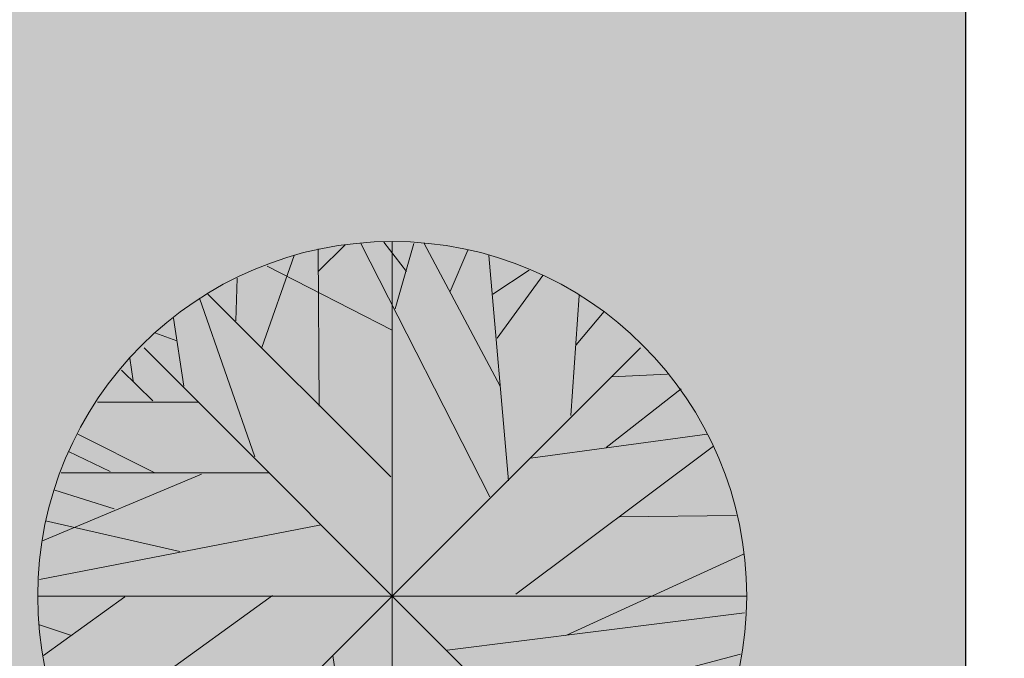
# Model space of a CAD drawing. Units: inches. Extents: x 459864 to 460310, y 324185 to 324787.
# Tile 74 of 112: x 460238 to 460271, y 324217 to 324238. Entities that reach past the tile are written whole.
import ezdxf

# ---------------------------------------------------------------- set-up
doc = ezdxf.new("R2010")
doc.units = ezdxf.units.IN
for name, color, linetype, lineweight in [('A-ANNO-DIMS', 2, 'Continuous', 18), ('C-PROP', 7, 'Continuous', 30), ('L-PLNT', 3, 'Continuous', 13), ('L-SITE-PATT', 252, 'Continuous', 13)]:
    doc.layers.add(name, color=color, linetype=linetype, lineweight=lineweight)
doc.styles.get("Standard").update_dxf_attribs({"font": 'arial.ttf'})
doc.dimstyles.new('ISO-25', dxfattribs={"dimtxt": 6, "dimasz": 2.5, "dimexe": 1.25, "dimexo": 0.625, "dimtad": 1, "dimdec": 1, "dimlunit": 3, "dimtxsty": 'Standard', "dimcen": 2.5, "dimadec": 0, "dimazin": 0, "dimtfac": 1, "dimtdec": 1, "dimtmove": 0, "dimatfit": 3, "dimfxl": 1, "dimarcsym": 0})

# ---------------------------------------------------------------- blocks, each defined once
blk = doc.blocks.new('Tree - deciduous plan')
for p, q in [((0, 59.9996), (0, -60)), ((-12.5388, 54.9406), (-7.9613, 59.4546)), ((-12.3627, 32.1443), (-12.5388, 58.7776)), ((-5.3205, 59.6806), (16.5105, 16.7963)), ((2.426, 54.9406), (-1.4472, 59.9056)), ((0.4894, 48.6208), (3.6584, 59.6806)), ((18.2711, 35.5298), (5.419, 59.6806)), ((9.8203, 51.5549), (12.8133, 58.5516)), ((-22.0458, 42.0753), (-16.5881, 57.6486)), ((19.6795, 19.5047), (16.3344, 57.6486)), ((-21.1656, 55.8436), (-0.0388, 45.0094)), ((17.0387, 51.1035), (23.2006, 55.1666)), ((-26.4472, 46.5894), (-26.2712, 53.8116)), ((17.7429, 43.6552), (25.4894, 54.2636)), ((-32.6092, 50.4264), (-23.2782, 23.5674)), ((-31.2008, 51.1035), (-0.2149, 20.1818)), ((31.6513, 50.8778), (30.2429, 30.5643)), ((-37.0107, 47.0408), (-35.25, 35.5298)), ((31.1232, 42.5267), (35.8767, 48.1693)), ((-40.1797, 44.558), (-36.4825, 43.2038)), ((42, 42), (-42, -42)), ((42, -42), (-42, 42)), ((-43.8768, 36.4326), (-44.405, 40.2696)), ((-45.8134, 38.2383), (-40.5318, 33.0471)), ((37.1091, 37.1098), (46.6161, 37.5612)), ((36.2288, 25.1474), (48.9049, 35.0784)), ((-49.8627, 32.8214), (-32.7853, 32.8214)), ((-53.2078, 27.4044), (-40.1797, 20.859)), ((23.3767, 23.3417), (53.3063, 27.4044)), ((54.3626, 25.3731), (20.9119, 0.3198)), ((-54.7923, 24.4702), (-47.75, 21.0847)), ((-32.2571, 20.6333), (-59.1937, 9.348)), ((-56.0247, 20.859), (-20.8134, 20.859)), ((-57.081, 17.9248), (-47.0458, 14.7649)), ((38.5175, 13.4107), (58.2359, 13.6364)), ((-59.7219, 2.8025), (-12.0106, 12.0565)), ((-58.6656, 12.7336), (-35.9543, 7.5424)), ((29.3626, -6.6771), (59.4682, 7.091)), ((-54.6162, -24.7335), (-20.2853, 0.0941)), ((-60, 0), (60, 0)), ((-45.2853, -0.1316), (-59.0177, -10.0627)), ((9.2922, -9.1598), (59.6443, -2.8401)), ((-59.7219, -4.8714), (-54.2641, -6.6771)), ((26.3697, -18.4138), (58.9401, -9.8369)), ((-10.074, -10.0627), (-2.5036, -59.7178))]:
    blk.add_line(p, q)
blk.add_circle((0, 0), 60)
blk = doc.blocks.new('*D65')
at = {"layer": 'A-ANNO-DIMS', "color": 0, "lineweight": -2, "transparency": 16777216}
for p, q in [((460247.74, 324283.483), (460302.765, 324283.483)), ((460301.515, 324280.983), (460301.515, 324197.483)), ((460271.74, 324194.983), (460302.765, 324194.983))]:
    blk.add_line(p, q, dxfattribs=at)
at = {"layer": 'A-ANNO-DIMS', "color": 0, "transparency": 16777216}
for points in [[(460301.098, 324280.983), (460301.932, 324280.983), (460301.515, 324283.483)], [(460301.098, 324197.483), (460301.932, 324197.483), (460301.515, 324194.983)]]:
    blk.add_solid(points, dxfattribs=at)
at = {"layer": 'Defpoints', "color": 0, "transparency": 16777216}
for p in [(460247.115, 324283.483), (460271.115, 324194.983), (460301.515, 324194.983)]:
    blk.add_point(p, dxfattribs=at)
at = {"layer": 'A-ANNO-DIMS', "color": 0, "transparency": 16777216, "insert": (460297.788, 324239.233), "char_height": 6, "attachment_point": 5, "rotation": 90}
blk.add_mtext('7\'-4 1/2"', dxfattribs=at)

msp = doc.modelspace()

# ---------------------------------------------------------------- hatches: boundary and pattern name
at = {"layer": 'L-SITE-PATT'}
h = msp.add_hatch(dxfattribs=at)
h.set_pattern_fill('DOTS', color=256)
h.paths.add_polyline_path([(460269.804, 324283.483), (460247.115, 324283.483), (460121.929, 324283.483), (460121.929, 324252.473), (460117.429, 324252.473), (460110.124, 324252.473), (460110.124, 324243.287), (460080.83, 324243.287), (460080.83, 324252.473), (460061.115, 324252.473), (460061.115, 324251.882), (460077.909, 324251.882), (460077.909, 324199.483), (460080.83, 324199.483), (460080.83, 324207.553), (460110.124, 324207.553), (460110.124, 324199.483), (460110.813, 324199.483), (460262.115, 324199.483), (460269.804, 324199.483)], flags=17)
edge = h.paths.add_edge_path(flags=0)
edge.add_ellipse((460222.59, 324263.813), major_axis=(-8.485, 8.485), ratio=1, start_angle=405, end_angle=495, ccw=False)
edge.add_line((460214.821, 324254.66), (460214.832, 324254.666))
edge.add_ellipse((460222.59, 324263.813), major_axis=(-8.485, 8.485), ratio=1, start_angle=405, end_angle=495, ccw=False)
edge.add_line((460210.759, 324261.781), (460210.768, 324261.787))
edge.add_ellipse((460222.59, 324263.813), major_axis=(-8.485, 8.485), ratio=1, start_angle=405, end_angle=495, ccw=False)
edge.add_ellipse((460222.59, 324263.813), major_axis=(-8.485, 8.485), ratio=1, start_angle=392.754, end_angle=405, ccw=False)
edge.add_ellipse((460222.59, 324263.813), major_axis=(-8.485, 8.485), ratio=1, start_angle=380.9347, end_angle=392.754, ccw=False)
edge.add_line((460211.337, 324267.985), (460211.34, 324267.985))
edge.add_ellipse((460222.59, 324263.813), major_axis=(-8.485, 8.485), ratio=1, start_angle=380.9347, end_angle=392.754, ccw=False)
edge.add_ellipse((460222.59, 324263.813), major_axis=(-8.485, 8.485), ratio=1, start_angle=347.9015, end_angle=380.9347, ccw=False)
edge.add_ellipse((460222.59, 324263.813), major_axis=(-8.485, 8.485), ratio=1, start_angle=327.0619, end_angle=347.9015, ccw=False)
edge.add_ellipse((460222.59, 324263.813), major_axis=(-8.485, 8.485), ratio=1, start_angle=278.3246, end_angle=327.0619, ccw=False)
edge.add_line((460225.158, 324275.536), (460225.158, 324275.535))
edge.add_ellipse((460222.59, 324263.813), major_axis=(-8.485, 8.485), ratio=1, start_angle=278.3246, end_angle=327.0619, ccw=False)
edge.add_ellipse((460222.59, 324263.813), major_axis=(-8.485, 8.485), ratio=1, start_angle=260.6436, end_angle=278.3246, ccw=False)
edge.add_ellipse((460222.59, 324263.813), major_axis=(-8.485, 8.485), ratio=1, start_angle=225, end_angle=260.6436, ccw=False)
edge.add_line((460234.509, 324265.243), (460234.501, 324265.239))
edge.add_ellipse((460222.59, 324263.813), major_axis=(-8.485, 8.485), ratio=1, start_angle=225, end_angle=260.6436, ccw=False)
edge.add_ellipse((460222.59, 324263.813), major_axis=(-8.485, 8.485), ratio=1, start_angle=495, end_angle=585, ccw=False)
edge.add_line((460234.437, 324261.861), (460234.424, 324261.858))
edge.add_ellipse((460222.59, 324263.813), major_axis=(-8.485, 8.485), ratio=1, start_angle=495, end_angle=585, ccw=False)
edge.add_line((460227.95, 324253.067), (460227.946, 324253.083))
edge.add_ellipse((460222.59, 324263.813), major_axis=(-8.485, 8.485), ratio=1, start_angle=495, end_angle=585, ccw=False)
edge.add_line((460226.223, 324252.369), (460226.211, 324252.38))
edge.add_ellipse((460222.59, 324263.813), major_axis=(-8.485, 8.485), ratio=1, start_angle=495, end_angle=585, ccw=False)
h.paths.add_polyline_path([(460219.651, 324254.347), (460218.461, 324253.545), (460218.275, 324254.789), (460219.642, 324256.542), (460219.625, 324260.848), (460216.11, 324257.333), (460214.35, 324256.978), (460215.416, 324259.356), (460212.524, 324258.496), (460213.137, 324259.93), (460218.507, 324263.813), (460222.59, 324263.813), (460222.59, 324267.807), (460218.176, 324272.212), (460219.026, 324274.639), (460222.59, 324272.811), (460222.59, 324275.423), (460223.057, 324274.825), (460222.675, 324273.492), (460225.912, 324267.135), (460219.625, 324260.848)], flags=0)
edge = h.paths.add_edge_path(flags=0)
edge.add_ellipse((460194.576, 324264.046), major_axis=(-8.485, 8.485), ratio=1, start_angle=495, end_angle=585, ccw=False)
edge.add_line((460199.936, 324253.3), (460199.932, 324253.316))
edge.add_ellipse((460194.576, 324264.046), major_axis=(-8.485, 8.485), ratio=1, start_angle=495, end_angle=585, ccw=False)
edge.add_line((460198.208, 324252.603), (460198.196, 324252.613))
edge.add_ellipse((460194.576, 324264.046), major_axis=(-8.485, 8.485), ratio=1, start_angle=495, end_angle=585, ccw=False)
edge.add_ellipse((460194.576, 324264.046), major_axis=(-8.485, 8.485), ratio=1, start_angle=405, end_angle=495, ccw=False)
edge.add_line((460186.806, 324254.893), (460186.817, 324254.899))
edge.add_ellipse((460194.576, 324264.046), major_axis=(-8.485, 8.485), ratio=1, start_angle=405, end_angle=495, ccw=False)
edge.add_line((460182.744, 324262.014), (460182.753, 324262.02))
edge.add_ellipse((460194.576, 324264.046), major_axis=(-8.485, 8.485), ratio=1, start_angle=405, end_angle=495, ccw=False)
edge.add_ellipse((460194.576, 324264.046), major_axis=(-8.485, 8.485), ratio=1, start_angle=392.754, end_angle=405, ccw=False)
edge.add_ellipse((460194.576, 324264.046), major_axis=(-8.485, 8.485), ratio=1, start_angle=380.9347, end_angle=392.754, ccw=False)
edge.add_line((460183.323, 324268.218), (460183.326, 324268.218))
edge.add_ellipse((460194.576, 324264.046), major_axis=(-8.485, 8.485), ratio=1, start_angle=380.9347, end_angle=392.754, ccw=False)
edge.add_ellipse((460194.576, 324264.046), major_axis=(-8.485, 8.485), ratio=1, start_angle=347.9015, end_angle=380.9347, ccw=False)
edge.add_ellipse((460194.576, 324264.046), major_axis=(-8.485, 8.485), ratio=1, start_angle=327.0619, end_angle=347.9015, ccw=False)
edge.add_ellipse((460194.576, 324264.046), major_axis=(-8.485, 8.485), ratio=1, start_angle=278.3246, end_angle=327.0619, ccw=False)
edge.add_line((460197.144, 324275.769), (460197.143, 324275.768))
edge.add_ellipse((460194.576, 324264.046), major_axis=(-8.485, 8.485), ratio=1, start_angle=278.3246, end_angle=327.0619, ccw=False)
edge.add_ellipse((460194.576, 324264.046), major_axis=(-8.485, 8.485), ratio=1, start_angle=260.6436, end_angle=278.3246, ccw=False)
edge.add_ellipse((460194.576, 324264.046), major_axis=(-8.485, 8.485), ratio=1, start_angle=225, end_angle=260.6436, ccw=False)
edge.add_line((460206.494, 324265.476), (460206.487, 324265.473))
edge.add_ellipse((460194.576, 324264.046), major_axis=(-8.485, 8.485), ratio=1, start_angle=225, end_angle=260.6436, ccw=False)
edge.add_ellipse((460194.576, 324264.046), major_axis=(-8.485, 8.485), ratio=1, start_angle=495, end_angle=585, ccw=False)
edge.add_line((460206.422, 324262.094), (460206.409, 324262.091))
h.paths.add_polyline_path([(460191.61, 324261.081), (460191.637, 324254.58), (460190.447, 324253.778), (460190.261, 324255.023), (460191.628, 324256.775), (460191.61, 324261.081), (460188.096, 324257.566), (460186.335, 324257.211), (460187.402, 324259.589), (460184.509, 324258.729), (460185.123, 324260.163), (460190.493, 324264.046), (460194.576, 324264.046), (460194.576, 324268.04), (460190.161, 324272.446), (460191.011, 324274.872), (460194.576, 324273.044), (460194.576, 324275.657), (460195.043, 324275.058), (460194.661, 324273.725), (460197.897, 324267.368)], flags=0)
edge = h.paths.add_edge_path(flags=0)
edge.add_ellipse((460252.912, 324263.578), major_axis=(-8.485, 8.485), ratio=1, start_angle=405, end_angle=495, ccw=False)
edge.add_line((460241.081, 324261.545), (460241.089, 324261.551))
edge.add_ellipse((460252.912, 324263.578), major_axis=(-8.485, 8.485), ratio=1, start_angle=405, end_angle=495, ccw=False)
edge.add_ellipse((460252.912, 324263.578), major_axis=(-8.485, 8.485), ratio=1, start_angle=392.754, end_angle=405, ccw=False)
edge.add_ellipse((460252.912, 324263.578), major_axis=(-8.485, 8.485), ratio=1, start_angle=380.9347, end_angle=392.754, ccw=False)
edge.add_line((460241.659, 324267.749), (460241.662, 324267.749))
edge.add_ellipse((460252.912, 324263.578), major_axis=(-8.485, 8.485), ratio=1, start_angle=380.9347, end_angle=392.754, ccw=False)
edge.add_ellipse((460252.912, 324263.578), major_axis=(-8.485, 8.485), ratio=1, start_angle=347.9015, end_angle=380.9347, ccw=False)
edge.add_ellipse((460252.912, 324263.578), major_axis=(-8.485, 8.485), ratio=1, start_angle=327.0619, end_angle=347.9015, ccw=False)
edge.add_ellipse((460252.912, 324263.578), major_axis=(-8.485, 8.485), ratio=1, start_angle=278.3246, end_angle=327.0619, ccw=False)
edge.add_line((460255.48, 324275.3), (460255.479, 324275.299))
edge.add_ellipse((460252.912, 324263.578), major_axis=(-8.485, 8.485), ratio=1, start_angle=278.3246, end_angle=327.0619, ccw=False)
edge.add_ellipse((460252.912, 324263.578), major_axis=(-8.485, 8.485), ratio=1, start_angle=260.6436, end_angle=278.3246, ccw=False)
edge.add_ellipse((460252.912, 324263.578), major_axis=(-8.485, 8.485), ratio=1, start_angle=225, end_angle=260.6436, ccw=False)
edge.add_line((460264.83, 324265.007), (460264.823, 324265.004))
edge.add_ellipse((460252.912, 324263.578), major_axis=(-8.485, 8.485), ratio=1, start_angle=225, end_angle=260.6436, ccw=False)
edge.add_ellipse((460252.912, 324263.578), major_axis=(-8.485, 8.485), ratio=1, start_angle=495, end_angle=585, ccw=False)
edge.add_line((460264.758, 324261.626), (460264.745, 324261.622))
edge.add_ellipse((460252.912, 324263.578), major_axis=(-8.485, 8.485), ratio=1, start_angle=495, end_angle=585, ccw=False)
edge.add_line((460258.272, 324252.832), (460258.268, 324252.848))
edge.add_ellipse((460252.912, 324263.578), major_axis=(-8.485, 8.485), ratio=1, start_angle=495, end_angle=585, ccw=False)
edge.add_line((460256.545, 324252.134), (460256.533, 324252.144))
edge.add_ellipse((460252.912, 324263.578), major_axis=(-8.485, 8.485), ratio=1, start_angle=495, end_angle=585, ccw=False)
edge.add_ellipse((460252.912, 324263.578), major_axis=(-8.485, 8.485), ratio=1, start_angle=405, end_angle=495, ccw=False)
edge.add_line((460245.143, 324254.424), (460245.153, 324254.43))
h.paths.add_polyline_path([(460244.672, 324256.742), (460245.738, 324259.12), (460242.846, 324258.26), (460243.459, 324259.694), (460248.829, 324263.578), (460252.912, 324263.578), (460252.912, 324267.571), (460248.497, 324271.977), (460249.348, 324274.403), (460252.912, 324272.576), (460252.912, 324275.188), (460253.379, 324274.589), (460252.997, 324273.257), (460256.233, 324266.899), (460249.946, 324260.612), (460249.973, 324254.111), (460248.783, 324253.309), (460248.597, 324254.554), (460249.964, 324256.306), (460249.946, 324260.612), (460246.432, 324257.097)], flags=0)
edge = h.paths.add_edge_path(flags=0)
edge.add_ellipse((460167.439, 324262.833), major_axis=(-8.485, 8.485), ratio=1, start_angle=495, end_angle=585, ccw=False)
edge.add_line((460172.799, 324252.087), (460172.795, 324252.103))
edge.add_ellipse((460167.439, 324262.833), major_axis=(-8.485, 8.485), ratio=1, start_angle=495, end_angle=585, ccw=False)
edge.add_line((460171.071, 324251.389), (460171.059, 324251.399))
edge.add_ellipse((460167.439, 324262.833), major_axis=(-8.485, 8.485), ratio=1, start_angle=495, end_angle=585, ccw=False)
edge.add_ellipse((460167.439, 324262.833), major_axis=(-8.485, 8.485), ratio=1, start_angle=405, end_angle=495, ccw=False)
edge.add_line((460159.669, 324253.679), (460159.68, 324253.685))
edge.add_ellipse((460167.439, 324262.833), major_axis=(-8.485, 8.485), ratio=1, start_angle=405, end_angle=495, ccw=False)
edge.add_line((460155.607, 324260.8), (460155.616, 324260.806))
edge.add_ellipse((460167.439, 324262.833), major_axis=(-8.485, 8.485), ratio=1, start_angle=405, end_angle=495, ccw=False)
edge.add_ellipse((460167.439, 324262.833), major_axis=(-8.485, 8.485), ratio=1, start_angle=392.754, end_angle=405, ccw=False)
edge.add_ellipse((460167.439, 324262.833), major_axis=(-8.485, 8.485), ratio=1, start_angle=380.9347, end_angle=392.754, ccw=False)
edge.add_line((460156.185, 324267.005), (460156.189, 324267.005))
edge.add_ellipse((460167.439, 324262.833), major_axis=(-8.485, 8.485), ratio=1, start_angle=380.9347, end_angle=392.754, ccw=False)
edge.add_ellipse((460167.439, 324262.833), major_axis=(-8.485, 8.485), ratio=1, start_angle=347.9015, end_angle=380.9347, ccw=False)
edge.add_ellipse((460167.439, 324262.833), major_axis=(-8.485, 8.485), ratio=1, start_angle=327.0619, end_angle=347.9015, ccw=False)
edge.add_ellipse((460167.439, 324262.833), major_axis=(-8.485, 8.485), ratio=1, start_angle=278.3246, end_angle=327.0619, ccw=False)
edge.add_line((460170.007, 324274.556), (460170.006, 324274.554))
edge.add_ellipse((460167.439, 324262.833), major_axis=(-8.485, 8.485), ratio=1, start_angle=278.3246, end_angle=327.0619, ccw=False)
edge.add_ellipse((460167.439, 324262.833), major_axis=(-8.485, 8.485), ratio=1, start_angle=260.6436, end_angle=278.3246, ccw=False)
edge.add_ellipse((460167.439, 324262.833), major_axis=(-8.485, 8.485), ratio=1, start_angle=225, end_angle=260.6436, ccw=False)
edge.add_line((460179.357, 324264.262), (460179.35, 324264.259))
edge.add_ellipse((460167.439, 324262.833), major_axis=(-8.485, 8.485), ratio=1, start_angle=225, end_angle=260.6436, ccw=False)
edge.add_ellipse((460167.439, 324262.833), major_axis=(-8.485, 8.485), ratio=1, start_angle=495, end_angle=585, ccw=False)
edge.add_line((460179.285, 324260.881), (460179.272, 324260.877))
h.paths.add_polyline_path([(460164.473, 324259.867), (460164.5, 324253.366), (460163.31, 324252.565), (460163.124, 324253.809), (460164.491, 324255.561), (460164.473, 324259.867), (460160.958, 324256.353), (460159.198, 324255.998), (460160.265, 324258.375), (460157.372, 324257.515), (460157.986, 324258.949), (460163.356, 324262.833), (460167.439, 324262.833), (460167.439, 324266.826), (460163.024, 324271.232), (460163.874, 324273.659), (460167.439, 324271.831), (460167.439, 324274.443), (460167.905, 324273.844), (460167.524, 324272.512), (460170.76, 324266.154)], flags=0)
edge = h.paths.add_edge_path(flags=0)
edge.add_ellipse((460140.758, 324262.37), major_axis=(-8.485, 8.485), ratio=1, start_angle=495, end_angle=585, ccw=False)
edge.add_line((460146.118, 324251.624), (460146.114, 324251.639))
edge.add_ellipse((460140.758, 324262.37), major_axis=(-8.485, 8.485), ratio=1, start_angle=495, end_angle=585, ccw=False)
edge.add_line((460144.391, 324250.926), (460144.379, 324250.936))
edge.add_ellipse((460140.758, 324262.37), major_axis=(-8.485, 8.485), ratio=1, start_angle=495, end_angle=585, ccw=False)
edge.add_ellipse((460140.758, 324262.37), major_axis=(-8.485, 8.485), ratio=1, start_angle=405, end_angle=495, ccw=False)
edge.add_line((460132.989, 324253.216), (460132.999, 324253.222))
edge.add_ellipse((460140.758, 324262.37), major_axis=(-8.485, 8.485), ratio=1, start_angle=405, end_angle=495, ccw=False)
edge.add_line((460128.927, 324260.337), (460128.935, 324260.343))
edge.add_ellipse((460140.758, 324262.37), major_axis=(-8.485, 8.485), ratio=1, start_angle=405, end_angle=495, ccw=False)
edge.add_ellipse((460140.758, 324262.37), major_axis=(-8.485, 8.485), ratio=1, start_angle=392.754, end_angle=405, ccw=False)
edge.add_ellipse((460140.758, 324262.37), major_axis=(-8.485, 8.485), ratio=1, start_angle=380.9347, end_angle=392.754, ccw=False)
edge.add_line((460129.505, 324266.541), (460129.508, 324266.541))
edge.add_ellipse((460140.758, 324262.37), major_axis=(-8.485, 8.485), ratio=1, start_angle=380.9347, end_angle=392.754, ccw=False)
edge.add_ellipse((460140.758, 324262.37), major_axis=(-8.485, 8.485), ratio=1, start_angle=347.9015, end_angle=380.9347, ccw=False)
edge.add_ellipse((460140.758, 324262.37), major_axis=(-8.485, 8.485), ratio=1, start_angle=327.0619, end_angle=347.9015, ccw=False)
edge.add_ellipse((460140.758, 324262.37), major_axis=(-8.485, 8.485), ratio=1, start_angle=278.3246, end_angle=327.0619, ccw=False)
edge.add_line((460143.326, 324274.092), (460143.325, 324274.091))
edge.add_ellipse((460140.758, 324262.37), major_axis=(-8.485, 8.485), ratio=1, start_angle=278.3246, end_angle=327.0619, ccw=False)
edge.add_ellipse((460140.758, 324262.37), major_axis=(-8.485, 8.485), ratio=1, start_angle=260.6436, end_angle=278.3246, ccw=False)
edge.add_ellipse((460140.758, 324262.37), major_axis=(-8.485, 8.485), ratio=1, start_angle=225, end_angle=260.6436, ccw=False)
edge.add_line((460152.677, 324263.799), (460152.669, 324263.796))
edge.add_ellipse((460140.758, 324262.37), major_axis=(-8.485, 8.485), ratio=1, start_angle=225, end_angle=260.6436, ccw=False)
edge.add_ellipse((460140.758, 324262.37), major_axis=(-8.485, 8.485), ratio=1, start_angle=495, end_angle=585, ccw=False)
edge.add_line((460152.604, 324260.418), (460152.592, 324260.414))
h.paths.add_polyline_path([(460137.792, 324259.404), (460137.819, 324252.903), (460136.629, 324252.101), (460136.443, 324253.346), (460137.81, 324255.098), (460137.792, 324259.404), (460134.278, 324255.889), (460132.518, 324255.534), (460133.584, 324257.912), (460130.692, 324257.052), (460131.305, 324258.486), (460136.675, 324262.37), (460140.758, 324262.37), (460140.758, 324266.363), (460136.343, 324270.769), (460137.194, 324273.195), (460140.758, 324271.367), (460140.758, 324273.98), (460141.225, 324273.381), (460140.843, 324272.049), (460144.079, 324265.691)], flags=0)
h.paths.add_polyline_path([(460110.124, 324227.414), (460080.83, 324227.414), (460080.83, 324235.484), (460110.124, 324235.484)], flags=16)
h.paths.add_polyline_path([(460110.124, 324220.797), (460110.124, 324212.727), (460080.83, 324212.727), (460080.83, 324220.797)], flags=16)
h.paths.add_polyline_path([(460269.804, 324283.483), (460247.115, 324283.483), (460121.929, 324283.483), (460121.929, 324252.473), (460117.429, 324252.473), (460110.124, 324252.473), (460110.124, 324243.287), (460080.83, 324243.287), (460080.83, 324252.473), (460061.115, 324252.473), (460061.115, 324251.882), (460077.909, 324251.882), (460077.909, 324199.483), (460080.83, 324199.483), (460080.83, 324207.553), (460110.124, 324207.553), (460110.124, 324199.483), (460262.115, 324199.483), (460269.804, 324199.483)], flags=17)
h.paths.add_polyline_path([(460219.651, 324254.347), (460218.461, 324253.545), (460218.275, 324254.789), (460219.642, 324256.542), (460219.625, 324260.848), (460216.11, 324257.333), (460214.35, 324256.978), (460215.416, 324259.356), (460212.524, 324258.496), (460213.137, 324259.93), (460218.507, 324263.813), (460222.59, 324263.813), (460220.18, 324266.223), (460215.461, 324265.308), (460211.835, 324266.137), (460216.247, 324267.985), (460218.418, 324267.985), (460222.59, 324263.813), (460222.59, 324267.807), (460218.176, 324272.212), (460219.026, 324274.639), (460222.59, 324272.811), (460222.59, 324275.423), (460223.057, 324274.825), (460222.675, 324273.492), (460225.912, 324267.135), (460222.59, 324263.813), (460231.383, 324263.813), (460228.485, 324262.488), (460224.425, 324261.978), (460228.68, 324257.724), (460228.966, 324254.791), (460227.142, 324256.537), (460227.542, 324254.819), (460227.333, 324253.614), (460222.59, 324259.985), (460222.59, 324255.497), (460221.377, 324256.541), (460220.576, 324261.799), (460219.625, 324260.848)], flags=0)
h.paths.add_polyline_path([(460199.127, 324256.77), (460199.528, 324255.052), (460199.319, 324253.848), (460194.576, 324260.218), (460194.576, 324255.73), (460193.363, 324256.774), (460192.561, 324262.032), (460191.61, 324261.081), (460191.637, 324254.58), (460190.447, 324253.778), (460190.261, 324255.023), (460191.628, 324256.775), (460191.61, 324261.081), (460188.096, 324257.566), (460186.335, 324257.211), (460187.402, 324259.589), (460184.509, 324258.729), (460185.123, 324260.163), (460190.493, 324264.046), (460194.576, 324264.046), (460192.166, 324266.456), (460187.446, 324265.541), (460183.82, 324266.37), (460188.232, 324268.218), (460190.404, 324268.218), (460194.576, 324264.046), (460194.576, 324268.04), (460190.161, 324272.446), (460191.011, 324274.872), (460194.576, 324273.044), (460194.576, 324275.657), (460195.043, 324275.058), (460194.661, 324273.725), (460197.897, 324267.368), (460194.576, 324264.046), (460203.368, 324264.046), (460200.47, 324262.721), (460196.411, 324262.212), (460200.665, 324257.957), (460200.951, 324255.024)], flags=0)
h.paths.add_polyline_path([(460244.672, 324256.742), (460245.738, 324259.12), (460242.846, 324258.26), (460243.459, 324259.694), (460248.829, 324263.578), (460252.912, 324263.578), (460250.502, 324265.987), (460245.783, 324265.072), (460242.156, 324265.901), (460246.568, 324267.749), (460248.74, 324267.749), (460252.912, 324263.578), (460252.912, 324267.571), (460248.497, 324271.977), (460249.348, 324274.403), (460252.912, 324272.576), (460252.912, 324275.188), (460253.379, 324274.589), (460252.997, 324273.257), (460256.233, 324266.899), (460252.912, 324263.578), (460261.705, 324263.578), (460258.806, 324262.252), (460254.747, 324261.743), (460259.002, 324257.488), (460259.288, 324254.555), (460257.463, 324256.301), (460257.864, 324254.583), (460257.655, 324253.379), (460252.912, 324259.749), (460252.912, 324255.261), (460251.699, 324256.305), (460250.897, 324261.563), (460249.946, 324260.612), (460249.973, 324254.111), (460248.783, 324253.309), (460248.597, 324254.554), (460249.964, 324256.306), (460249.946, 324260.612), (460246.432, 324257.097)], flags=0)
h.paths.add_polyline_path([(460173.528, 324256.743), (460173.814, 324253.811), (460171.99, 324255.556), (460172.39, 324253.838), (460172.182, 324252.634), (460167.439, 324259.004), (460167.439, 324254.516), (460166.226, 324255.56), (460165.424, 324260.818), (460164.473, 324259.867), (460164.5, 324253.366), (460163.31, 324252.565), (460163.124, 324253.809), (460164.491, 324255.561), (460164.473, 324259.867), (460160.958, 324256.353), (460159.198, 324255.998), (460160.265, 324258.375), (460157.372, 324257.515), (460157.986, 324258.949), (460163.356, 324262.833), (460167.439, 324262.833), (460165.029, 324265.243), (460160.309, 324264.327), (460156.683, 324265.156), (460161.095, 324267.005), (460163.267, 324267.005), (460167.439, 324262.833), (460167.439, 324266.826), (460163.024, 324271.232), (460163.874, 324273.659), (460167.439, 324271.831), (460167.439, 324274.443), (460167.905, 324273.844), (460167.524, 324272.512), (460170.76, 324266.154), (460167.439, 324262.833), (460176.231, 324262.833), (460173.333, 324261.507), (460169.274, 324260.998)], flags=0)
h.paths.add_polyline_path([(460146.848, 324256.28), (460147.134, 324253.347), (460145.31, 324255.093), (460145.71, 324253.375), (460145.501, 324252.171), (460140.758, 324258.541), (460140.758, 324254.053), (460139.545, 324255.097), (460138.744, 324260.355), (460137.792, 324259.404), (460137.819, 324252.903), (460136.629, 324252.101), (460136.443, 324253.346), (460137.81, 324255.098), (460137.792, 324259.404), (460134.278, 324255.889), (460132.518, 324255.534), (460133.584, 324257.912), (460130.692, 324257.052), (460131.305, 324258.486), (460136.675, 324262.37), (460140.758, 324262.37), (460138.348, 324264.779), (460133.629, 324263.864), (460130.002, 324264.693), (460134.414, 324266.541), (460136.586, 324266.541), (460140.758, 324262.37), (460140.758, 324266.363), (460136.343, 324270.769), (460137.194, 324273.195), (460140.758, 324271.367), (460140.758, 324273.98), (460141.225, 324273.381), (460140.843, 324272.049), (460144.079, 324265.691), (460140.758, 324262.37), (460149.551, 324262.37), (460146.653, 324261.044), (460142.593, 324260.535)], flags=0)
edge = h.paths.add_edge_path()
edge.add_line((460269.804, 324272.549), (460260.881, 324272.549))
edge.add_ellipse((460252.912, 324263.578), major_axis=(-8.485, 8.485), ratio=1, start_angle=260.6436, end_angle=273.3846, ccw=False)
edge.add_line((460262.283, 324271.092), (460262.261, 324271.091))
edge.add_ellipse((460252.912, 324263.578), major_axis=(-8.485, 8.485), ratio=1, start_angle=260.6436, end_angle=273.3846, ccw=False)
edge.add_ellipse((460252.912, 324263.578), major_axis=(-8.485, 8.485), ratio=1, start_angle=225, end_angle=260.6436, ccw=False)
edge.add_line((460263.609, 324269.063), (460263.572, 324269.058))
edge.add_ellipse((460252.912, 324263.578), major_axis=(-8.485, 8.485), ratio=1, start_angle=225, end_angle=260.6436, ccw=False)
edge.add_line((460264.615, 324266.306), (460264.585, 324266.305))
edge.add_ellipse((460252.912, 324263.578), major_axis=(-8.485, 8.485), ratio=1, start_angle=225, end_angle=260.6436, ccw=False)
edge.add_line((460264.83, 324265.007), (460264.823, 324265.004))
edge.add_ellipse((460252.912, 324263.578), major_axis=(-8.485, 8.485), ratio=1, start_angle=225, end_angle=260.6436, ccw=False)
edge.add_ellipse((460252.912, 324263.578), major_axis=(-8.485, 8.485), ratio=1, start_angle=495, end_angle=585, ccw=False)
edge.add_line((460264.758, 324261.626), (460264.745, 324261.622))
edge.add_ellipse((460252.912, 324263.578), major_axis=(-8.485, 8.485), ratio=1, start_angle=495, end_angle=585, ccw=False)
edge.add_line((460263.442, 324257.739), (460263.389, 324257.779))
edge.add_ellipse((460252.912, 324263.578), major_axis=(-8.485, 8.485), ratio=1, start_angle=495, end_angle=585, ccw=False)
edge.add_line((460258.128, 324252.744), (460258.102, 324252.779))
edge.add_ellipse((460252.912, 324263.578), major_axis=(-8.485, 8.485), ratio=1, start_angle=495, end_angle=585, ccw=False)
edge.add_line((460256.545, 324252.134), (460256.533, 324252.144))
edge.add_ellipse((460252.912, 324263.578), major_axis=(-8.485, 8.485), ratio=1, start_angle=495, end_angle=585, ccw=False)
edge.add_ellipse((460252.912, 324263.578), major_axis=(-8.485, 8.485), ratio=1, start_angle=405, end_angle=495, ccw=False)
edge.add_line((460250.594, 324251.78), (460250.605, 324251.82))
edge.add_ellipse((460252.912, 324263.578), major_axis=(-8.485, 8.485), ratio=1, start_angle=405, end_angle=495, ccw=False)
edge.add_line((460245.143, 324254.424), (460245.153, 324254.43))
edge.add_ellipse((460252.912, 324263.578), major_axis=(-8.485, 8.485), ratio=1, start_angle=405, end_angle=495, ccw=False)
edge.add_line((460243.525, 324256.059), (460243.56, 324256.091))
edge.add_ellipse((460252.912, 324263.578), major_axis=(-8.485, 8.485), ratio=1, start_angle=405, end_angle=495, ccw=False)
edge.add_line((460241.44, 324259.893), (460241.522, 324259.896))
edge.add_ellipse((460252.912, 324263.578), major_axis=(-8.485, 8.485), ratio=1, start_angle=405, end_angle=495, ccw=False)
edge.add_line((460241.081, 324261.545), (460241.089, 324261.551))
edge.add_ellipse((460252.912, 324263.578), major_axis=(-8.485, 8.485), ratio=1, start_angle=405, end_angle=495, ccw=False)
edge.add_ellipse((460252.912, 324263.578), major_axis=(-8.485, 8.485), ratio=1, start_angle=392.754, end_angle=405, ccw=False)
edge.add_line((460241.05, 324265.438), (460241.063, 324265.443))
edge.add_ellipse((460252.912, 324263.578), major_axis=(-8.485, 8.485), ratio=1, start_angle=392.754, end_angle=405, ccw=False)
edge.add_ellipse((460252.912, 324263.578), major_axis=(-8.485, 8.485), ratio=1, start_angle=380.9347, end_angle=392.754, ccw=False)
edge.add_line((460241.452, 324267.176), (460241.469, 324267.171))
edge.add_ellipse((460252.912, 324263.578), major_axis=(-8.485, 8.485), ratio=1, start_angle=380.9347, end_angle=392.754, ccw=False)
edge.add_line((460241.659, 324267.749), (460241.662, 324267.749))
edge.add_ellipse((460252.912, 324263.578), major_axis=(-8.485, 8.485), ratio=1, start_angle=380.9347, end_angle=392.754, ccw=False)
edge.add_ellipse((460252.912, 324263.578), major_axis=(-8.485, 8.485), ratio=1, start_angle=356.6154, end_angle=380.9347, ccw=False)
edge.add_line((460244.88, 324272.488), (460244.713, 324272.549))
edge.add_line((460244.713, 324272.549), (460230.817, 324272.549))
edge.add_ellipse((460222.59, 324263.813), major_axis=(-8.485, 8.485), ratio=1, start_angle=260.6436, end_angle=271.7178, ccw=False)
edge.add_ellipse((460222.59, 324263.813), major_axis=(-8.485, 8.485), ratio=1, start_angle=225, end_angle=260.6436, ccw=False)
edge.add_line((460233.287, 324269.299), (460233.25, 324269.294))
edge.add_ellipse((460222.59, 324263.813), major_axis=(-8.485, 8.485), ratio=1, start_angle=225, end_angle=260.6436, ccw=False)
edge.add_line((460234.294, 324266.541), (460234.264, 324266.541))
edge.add_ellipse((460222.59, 324263.813), major_axis=(-8.485, 8.485), ratio=1, start_angle=225, end_angle=260.6436, ccw=False)
edge.add_line((460234.509, 324265.243), (460234.501, 324265.239))
edge.add_ellipse((460222.59, 324263.813), major_axis=(-8.485, 8.485), ratio=1, start_angle=225, end_angle=260.6436, ccw=False)
edge.add_ellipse((460222.59, 324263.813), major_axis=(-8.485, 8.485), ratio=1, start_angle=495, end_angle=585, ccw=False)
edge.add_line((460234.437, 324261.861), (460234.424, 324261.858))
edge.add_ellipse((460222.59, 324263.813), major_axis=(-8.485, 8.485), ratio=1, start_angle=495, end_angle=585, ccw=False)
edge.add_line((460233.121, 324257.975), (460233.068, 324258.015))
edge.add_ellipse((460222.59, 324263.813), major_axis=(-8.485, 8.485), ratio=1, start_angle=495, end_angle=585, ccw=False)
edge.add_line((460227.806, 324252.979), (460227.78, 324253.014))
edge.add_ellipse((460222.59, 324263.813), major_axis=(-8.485, 8.485), ratio=1, start_angle=495, end_angle=585, ccw=False)
edge.add_line((460226.223, 324252.369), (460226.211, 324252.38))
edge.add_ellipse((460222.59, 324263.813), major_axis=(-8.485, 8.485), ratio=1, start_angle=495, end_angle=585, ccw=False)
edge.add_ellipse((460222.59, 324263.813), major_axis=(-8.485, 8.485), ratio=1, start_angle=405, end_angle=495, ccw=False)
edge.add_line((460220.272, 324252.016), (460220.283, 324252.055))
edge.add_ellipse((460222.59, 324263.813), major_axis=(-8.485, 8.485), ratio=1, start_angle=405, end_angle=495, ccw=False)
edge.add_line((460214.821, 324254.66), (460214.832, 324254.666))
edge.add_ellipse((460222.59, 324263.813), major_axis=(-8.485, 8.485), ratio=1, start_angle=405, end_angle=495, ccw=False)
edge.add_line((460213.203, 324256.295), (460213.239, 324256.327))
edge.add_ellipse((460222.59, 324263.813), major_axis=(-8.485, 8.485), ratio=1, start_angle=405, end_angle=495, ccw=False)
edge.add_line((460211.118, 324260.128), (460211.201, 324260.131))
edge.add_ellipse((460222.59, 324263.813), major_axis=(-8.485, 8.485), ratio=1, start_angle=405, end_angle=495, ccw=False)
edge.add_line((460210.759, 324261.781), (460210.768, 324261.787))
edge.add_ellipse((460222.59, 324263.813), major_axis=(-8.485, 8.485), ratio=1, start_angle=405, end_angle=495, ccw=False)
edge.add_ellipse((460222.59, 324263.813), major_axis=(-8.485, 8.485), ratio=1, start_angle=392.754, end_angle=405, ccw=False)
edge.add_line((460210.729, 324265.673), (460210.741, 324265.678))
edge.add_ellipse((460222.59, 324263.813), major_axis=(-8.485, 8.485), ratio=1, start_angle=392.754, end_angle=405, ccw=False)
edge.add_ellipse((460222.59, 324263.813), major_axis=(-8.485, 8.485), ratio=1, start_angle=380.9347, end_angle=392.754, ccw=False)
edge.add_line((460211.13, 324267.412), (460211.147, 324267.407))
edge.add_ellipse((460222.59, 324263.813), major_axis=(-8.485, 8.485), ratio=1, start_angle=380.9347, end_angle=392.754, ccw=False)
edge.add_line((460211.337, 324267.985), (460211.34, 324267.985))
edge.add_ellipse((460222.59, 324263.813), major_axis=(-8.485, 8.485), ratio=1, start_angle=380.9347, end_angle=392.754, ccw=False)
edge.add_ellipse((460222.59, 324263.813), major_axis=(-8.485, 8.485), ratio=1, start_angle=358.2822, end_angle=380.9347, ccw=False)
edge.add_line((460213.705, 324271.902), (460213.709, 324271.869))
edge.add_ellipse((460222.59, 324263.813), major_axis=(-8.485, 8.485), ratio=1, start_angle=358.2822, end_angle=380.9347, ccw=False)
edge.add_line((460214.363, 324272.549), (460203.078, 324272.549))
edge.add_line((460203.078, 324272.549), (460203.06, 324272.531))
edge.add_ellipse((460194.576, 324264.046), major_axis=(-8.485, 8.485), ratio=1, start_angle=260.6436, end_angle=270.1168, ccw=False)
edge.add_line((460203.957, 324271.561), (460203.921, 324271.56))
edge.add_ellipse((460194.576, 324264.046), major_axis=(-8.485, 8.485), ratio=1, start_angle=260.6436, end_angle=270.1168, ccw=False)
edge.add_ellipse((460194.576, 324264.046), major_axis=(-8.485, 8.485), ratio=1, start_angle=225, end_angle=260.6436, ccw=False)
edge.add_line((460205.272, 324269.532), (460205.235, 324269.527))
edge.add_ellipse((460194.576, 324264.046), major_axis=(-8.485, 8.485), ratio=1, start_angle=225, end_angle=260.6436, ccw=False)
edge.add_line((460206.279, 324266.774), (460206.249, 324266.774))
edge.add_ellipse((460194.576, 324264.046), major_axis=(-8.485, 8.485), ratio=1, start_angle=225, end_angle=260.6436, ccw=False)
edge.add_line((460206.494, 324265.476), (460206.487, 324265.473))
edge.add_ellipse((460194.576, 324264.046), major_axis=(-8.485, 8.485), ratio=1, start_angle=225, end_angle=260.6436, ccw=False)
edge.add_ellipse((460194.576, 324264.046), major_axis=(-8.485, 8.485), ratio=1, start_angle=495, end_angle=585, ccw=False)
edge.add_line((460206.422, 324262.094), (460206.409, 324262.091))
edge.add_ellipse((460194.576, 324264.046), major_axis=(-8.485, 8.485), ratio=1, start_angle=495, end_angle=585, ccw=False)
edge.add_line((460205.106, 324258.208), (460205.053, 324258.248))
edge.add_ellipse((460194.576, 324264.046), major_axis=(-8.485, 8.485), ratio=1, start_angle=495, end_angle=585, ccw=False)
edge.add_line((460199.792, 324253.212), (460199.766, 324253.248))
edge.add_ellipse((460194.576, 324264.046), major_axis=(-8.485, 8.485), ratio=1, start_angle=495, end_angle=585, ccw=False)
edge.add_line((460198.208, 324252.603), (460198.196, 324252.613))
edge.add_ellipse((460194.576, 324264.046), major_axis=(-8.485, 8.485), ratio=1, start_angle=495, end_angle=585, ccw=False)
edge.add_ellipse((460194.576, 324264.046), major_axis=(-8.485, 8.485), ratio=1, start_angle=405, end_angle=495, ccw=False)
edge.add_line((460192.258, 324252.249), (460192.268, 324252.289))
edge.add_ellipse((460194.576, 324264.046), major_axis=(-8.485, 8.485), ratio=1, start_angle=405, end_angle=495, ccw=False)
edge.add_line((460186.806, 324254.893), (460186.817, 324254.899))
edge.add_ellipse((460194.576, 324264.046), major_axis=(-8.485, 8.485), ratio=1, start_angle=405, end_angle=495, ccw=False)
edge.add_line((460185.188, 324256.528), (460185.224, 324256.56))
edge.add_ellipse((460194.576, 324264.046), major_axis=(-8.485, 8.485), ratio=1, start_angle=405, end_angle=495, ccw=False)
edge.add_line((460183.104, 324260.362), (460183.186, 324260.365))
edge.add_ellipse((460194.576, 324264.046), major_axis=(-8.485, 8.485), ratio=1, start_angle=405, end_angle=495, ccw=False)
edge.add_line((460182.744, 324262.014), (460182.753, 324262.02))
edge.add_ellipse((460194.576, 324264.046), major_axis=(-8.485, 8.485), ratio=1, start_angle=405, end_angle=495, ccw=False)
edge.add_ellipse((460194.576, 324264.046), major_axis=(-8.485, 8.485), ratio=1, start_angle=392.754, end_angle=405, ccw=False)
edge.add_line((460182.714, 324265.906), (460182.726, 324265.912))
edge.add_ellipse((460194.576, 324264.046), major_axis=(-8.485, 8.485), ratio=1, start_angle=392.754, end_angle=405, ccw=False)
edge.add_ellipse((460194.576, 324264.046), major_axis=(-8.485, 8.485), ratio=1, start_angle=380.9347, end_angle=392.754, ccw=False)
edge.add_line((460183.116, 324267.645), (460183.133, 324267.64))
edge.add_ellipse((460194.576, 324264.046), major_axis=(-8.485, 8.485), ratio=1, start_angle=380.9347, end_angle=392.754, ccw=False)
edge.add_line((460183.323, 324268.218), (460183.326, 324268.218))
edge.add_ellipse((460194.576, 324264.046), major_axis=(-8.485, 8.485), ratio=1, start_angle=380.9347, end_angle=392.754, ccw=False)
edge.add_ellipse((460194.576, 324264.046), major_axis=(-8.485, 8.485), ratio=1, start_angle=359.8832, end_angle=380.9347, ccw=False)
edge.add_line((460184.491, 324270.611), (460184.553, 324270.611))
edge.add_ellipse((460194.576, 324264.046), major_axis=(-8.485, 8.485), ratio=1, start_angle=359.8832, end_angle=380.9347, ccw=False)
edge.add_line((460185.346, 324271.76), (460185.379, 324271.728))
edge.add_ellipse((460194.576, 324264.046), major_axis=(-8.485, 8.485), ratio=1, start_angle=359.8832, end_angle=380.9347, ccw=False)
edge.add_line((460185.697, 324272.086), (460185.633, 324272.549))
edge.add_line((460185.633, 324272.549), (460174.683, 324272.549))
edge.add_line((460174.683, 324272.549), (460174.606, 324272.457))
edge.add_ellipse((460167.439, 324262.833), major_axis=(-8.485, 8.485), ratio=1, start_angle=260.6436, end_angle=278.3246, ccw=False)
edge.add_ellipse((460167.439, 324262.833), major_axis=(-8.485, 8.485), ratio=1, start_angle=225, end_angle=260.6436, ccw=False)
edge.add_line((460178.135, 324268.318), (460178.098, 324268.313))
edge.add_ellipse((460167.439, 324262.833), major_axis=(-8.485, 8.485), ratio=1, start_angle=225, end_angle=260.6436, ccw=False)
edge.add_line((460179.142, 324265.561), (460179.112, 324265.56))
edge.add_ellipse((460167.439, 324262.833), major_axis=(-8.485, 8.485), ratio=1, start_angle=225, end_angle=260.6436, ccw=False)
edge.add_line((460179.357, 324264.262), (460179.35, 324264.259))
edge.add_ellipse((460167.439, 324262.833), major_axis=(-8.485, 8.485), ratio=1, start_angle=225, end_angle=260.6436, ccw=False)
edge.add_ellipse((460167.439, 324262.833), major_axis=(-8.485, 8.485), ratio=1, start_angle=495, end_angle=585, ccw=False)
edge.add_line((460179.285, 324260.881), (460179.272, 324260.877))
edge.add_ellipse((460167.439, 324262.833), major_axis=(-8.485, 8.485), ratio=1, start_angle=495, end_angle=585, ccw=False)
edge.add_line((460177.969, 324256.994), (460177.916, 324257.034))
edge.add_ellipse((460167.439, 324262.833), major_axis=(-8.485, 8.485), ratio=1, start_angle=495, end_angle=585, ccw=False)
edge.add_line((460172.655, 324251.999), (460172.629, 324252.034))
edge.add_ellipse((460167.439, 324262.833), major_axis=(-8.485, 8.485), ratio=1, start_angle=495, end_angle=585, ccw=False)
edge.add_line((460171.071, 324251.389), (460171.059, 324251.399))
edge.add_ellipse((460167.439, 324262.833), major_axis=(-8.485, 8.485), ratio=1, start_angle=495, end_angle=585, ccw=False)
edge.add_ellipse((460167.439, 324262.833), major_axis=(-8.485, 8.485), ratio=1, start_angle=405, end_angle=495, ccw=False)
edge.add_line((460165.121, 324251.036), (460165.131, 324251.075))
edge.add_ellipse((460167.439, 324262.833), major_axis=(-8.485, 8.485), ratio=1, start_angle=405, end_angle=495, ccw=False)
edge.add_line((460159.669, 324253.679), (460159.68, 324253.685))
edge.add_ellipse((460167.439, 324262.833), major_axis=(-8.485, 8.485), ratio=1, start_angle=405, end_angle=495, ccw=False)
edge.add_line((460158.051, 324255.314), (460158.087, 324255.347))
edge.add_ellipse((460167.439, 324262.833), major_axis=(-8.485, 8.485), ratio=1, start_angle=405, end_angle=495, ccw=False)
edge.add_line((460155.967, 324259.148), (460156.049, 324259.151))
edge.add_ellipse((460167.439, 324262.833), major_axis=(-8.485, 8.485), ratio=1, start_angle=405, end_angle=495, ccw=False)
edge.add_line((460155.607, 324260.8), (460155.616, 324260.806))
edge.add_ellipse((460167.439, 324262.833), major_axis=(-8.485, 8.485), ratio=1, start_angle=405, end_angle=495, ccw=False)
edge.add_ellipse((460167.439, 324262.833), major_axis=(-8.485, 8.485), ratio=1, start_angle=392.754, end_angle=405, ccw=False)
edge.add_line((460155.577, 324264.693), (460155.589, 324264.698))
edge.add_ellipse((460167.439, 324262.833), major_axis=(-8.485, 8.485), ratio=1, start_angle=392.754, end_angle=405, ccw=False)
edge.add_ellipse((460167.439, 324262.833), major_axis=(-8.485, 8.485), ratio=1, start_angle=380.9347, end_angle=392.754, ccw=False)
edge.add_line((460155.979, 324266.432), (460155.996, 324266.426))
edge.add_ellipse((460167.439, 324262.833), major_axis=(-8.485, 8.485), ratio=1, start_angle=380.9347, end_angle=392.754, ccw=False)
edge.add_line((460156.185, 324267.005), (460156.189, 324267.005))
edge.add_ellipse((460167.439, 324262.833), major_axis=(-8.485, 8.485), ratio=1, start_angle=380.9347, end_angle=392.754, ccw=False)
edge.add_ellipse((460167.439, 324262.833), major_axis=(-8.485, 8.485), ratio=1, start_angle=350.9345, end_angle=380.9347, ccw=False)
edge.add_line((460157.363, 324269.397), (460157.414, 324269.397))
edge.add_ellipse((460167.439, 324262.833), major_axis=(-8.485, 8.485), ratio=1, start_angle=350.9345, end_angle=380.9347, ccw=False)
edge.add_line((460158.221, 324270.535), (460158.236, 324270.519))
edge.add_ellipse((460167.439, 324262.833), major_axis=(-8.485, 8.485), ratio=1, start_angle=350.9345, end_angle=380.9347, ccw=False)
edge.add_line((460159.379, 324271.753), (460159.419, 324271.738))
edge.add_ellipse((460167.439, 324262.833), major_axis=(-8.485, 8.485), ratio=1, start_angle=350.9345, end_angle=380.9347, ccw=False)
edge.add_line((460160.396, 324272.549), (460147.112, 324272.549))
edge.add_ellipse((460140.758, 324262.37), major_axis=(-8.485, 8.485), ratio=1, start_angle=278.3246, end_angle=283.0261, ccw=False)
edge.add_ellipse((460140.758, 324262.37), major_axis=(-8.485, 8.485), ratio=1, start_angle=260.6436, end_angle=278.3246, ccw=False)
edge.add_ellipse((460140.758, 324262.37), major_axis=(-8.485, 8.485), ratio=1, start_angle=225, end_angle=260.6436, ccw=False)
edge.add_line((460151.455, 324267.855), (460151.418, 324267.85))
edge.add_ellipse((460140.758, 324262.37), major_axis=(-8.485, 8.485), ratio=1, start_angle=225, end_angle=260.6436, ccw=False)
edge.add_line((460152.462, 324265.098), (460152.431, 324265.097))
edge.add_ellipse((460140.758, 324262.37), major_axis=(-8.485, 8.485), ratio=1, start_angle=225, end_angle=260.6436, ccw=False)
edge.add_line((460152.677, 324263.799), (460152.669, 324263.796))
edge.add_ellipse((460140.758, 324262.37), major_axis=(-8.485, 8.485), ratio=1, start_angle=225, end_angle=260.6436, ccw=False)
edge.add_ellipse((460140.758, 324262.37), major_axis=(-8.485, 8.485), ratio=1, start_angle=495, end_angle=585, ccw=False)
edge.add_line((460152.604, 324260.418), (460152.592, 324260.414))
edge.add_ellipse((460140.758, 324262.37), major_axis=(-8.485, 8.485), ratio=1, start_angle=495, end_angle=585, ccw=False)
edge.add_line((460151.288, 324256.531), (460151.235, 324256.571))
edge.add_ellipse((460140.758, 324262.37), major_axis=(-8.485, 8.485), ratio=1, start_angle=495, end_angle=585, ccw=False)
edge.add_line((460145.974, 324251.535), (460145.948, 324251.571))
edge.add_ellipse((460140.758, 324262.37), major_axis=(-8.485, 8.485), ratio=1, start_angle=495, end_angle=585, ccw=False)
edge.add_line((460144.391, 324250.926), (460144.379, 324250.936))
edge.add_ellipse((460140.758, 324262.37), major_axis=(-8.485, 8.485), ratio=1, start_angle=495, end_angle=585, ccw=False)
edge.add_ellipse((460140.758, 324262.37), major_axis=(-8.485, 8.485), ratio=1, start_angle=405, end_angle=495, ccw=False)
edge.add_line((460138.44, 324250.572), (460138.451, 324250.612))
edge.add_ellipse((460140.758, 324262.37), major_axis=(-8.485, 8.485), ratio=1, start_angle=405, end_angle=495, ccw=False)
edge.add_line((460132.989, 324253.216), (460132.999, 324253.222))
edge.add_ellipse((460140.758, 324262.37), major_axis=(-8.485, 8.485), ratio=1, start_angle=405, end_angle=495, ccw=False)
edge.add_line((460131.371, 324254.851), (460131.406, 324254.883))
edge.add_ellipse((460140.758, 324262.37), major_axis=(-8.485, 8.485), ratio=1, start_angle=405, end_angle=495, ccw=False)
edge.add_line((460129.286, 324258.685), (460129.369, 324258.688))
edge.add_ellipse((460140.758, 324262.37), major_axis=(-8.485, 8.485), ratio=1, start_angle=405, end_angle=495, ccw=False)
edge.add_line((460128.927, 324260.337), (460128.935, 324260.343))
edge.add_ellipse((460140.758, 324262.37), major_axis=(-8.485, 8.485), ratio=1, start_angle=405, end_angle=495, ccw=False)
edge.add_ellipse((460140.758, 324262.37), major_axis=(-8.485, 8.485), ratio=1, start_angle=392.754, end_angle=405, ccw=False)
edge.add_line((460128.896, 324264.23), (460128.909, 324264.235))
edge.add_ellipse((460140.758, 324262.37), major_axis=(-8.485, 8.485), ratio=1, start_angle=392.754, end_angle=405, ccw=False)
edge.add_ellipse((460140.758, 324262.37), major_axis=(-8.485, 8.485), ratio=1, start_angle=380.9347, end_angle=392.754, ccw=False)
edge.add_line((460129.298, 324265.968), (460129.315, 324265.963))
edge.add_ellipse((460140.758, 324262.37), major_axis=(-8.485, 8.485), ratio=1, start_angle=380.9347, end_angle=392.754, ccw=False)
edge.add_line((460129.505, 324266.541), (460129.508, 324266.541))
edge.add_ellipse((460140.758, 324262.37), major_axis=(-8.485, 8.485), ratio=1, start_angle=380.9347, end_angle=392.754, ccw=False)
edge.add_ellipse((460140.758, 324262.37), major_axis=(-8.485, 8.485), ratio=1, start_angle=347.9015, end_angle=380.9347, ccw=False)
edge.add_line((460130.697, 324268.934), (460130.727, 324268.934))
edge.add_ellipse((460140.758, 324262.37), major_axis=(-8.485, 8.485), ratio=1, start_angle=347.9015, end_angle=380.9347, ccw=False)
edge.add_line((460131.869, 324270.48), (460131.879, 324270.413))
edge.add_ellipse((460140.758, 324262.37), major_axis=(-8.485, 8.485), ratio=1, start_angle=347.9015, end_angle=380.9347, ccw=False)
edge.add_line((460132.734, 324271.277), (460132.705, 324271.287))
edge.add_ellipse((460140.758, 324262.37), major_axis=(-8.485, 8.485), ratio=1, start_angle=347.9015, end_angle=380.9347, ccw=False)
edge.add_line((460134.24, 324272.445), (460134.204, 324272.549))
edge.add_line((460134.204, 324272.549), (460121.929, 324272.549))
edge.add_line((460121.929, 324272.549), (460121.929, 324252.473))
edge.add_line((460121.929, 324252.473), (460117.429, 324252.473))
edge.add_line((460117.429, 324252.473), (460110.124, 324252.473))
edge.add_line((460110.124, 324252.473), (460110.124, 324243.287))
edge.add_line((460110.124, 324243.287), (460080.83, 324243.287))
edge.add_line((460080.83, 324243.287), (460080.83, 324252.473))
edge.add_line((460080.83, 324252.473), (460061.115, 324252.473))
edge.add_line((460061.115, 324252.473), (460061.115, 324251.882))
edge.add_line((460061.115, 324251.882), (460077.909, 324251.882))
edge.add_line((460077.909, 324251.882), (460077.909, 324199.483))
edge.add_line((460077.909, 324199.483), (460080.83, 324199.483))
edge.add_line((460080.83, 324199.483), (460080.83, 324207.553))
edge.add_line((460080.83, 324207.553), (460110.124, 324207.553))
edge.add_line((460110.124, 324207.553), (460110.124, 324199.483))
edge.add_line((460110.124, 324199.483), (460110.813, 324199.483))
edge.add_line((460110.813, 324199.483), (460262.115, 324199.483))
edge.add_line((460262.115, 324199.483), (460269.804, 324199.483))
edge.add_line((460269.804, 324199.483), (460269.804, 324272.549))

# ---------------------------------------------------------------- linework, layer by layer
at = {"layer": 'C-PROP'}
msp.add_line((460269.804, 324466.483), (460269.804, 324199.483), dxfattribs=at)

# ---------------------------------------------------------------- block references
at = {"layer": 'L-PLNT', "xscale": 0.2, "yscale": 0.2}
msp.add_blockref('Tree - deciduous plan', (460250.396, 324218.703), dxfattribs=at)

# ---------------------------------------------------------------- dimensions: what is measured, and where the dimension line sits
at = {"layer": 'A-ANNO-DIMS'}
dim = msp.add_linear_dim(base=(460301.515, 324194.983), p1=(460247.115, 324283.483), p2=(460271.115, 324194.983), angle=90, dimstyle='ISO-25', override={"dimdec": 1, "dimlfac": 1, "dimrnd": 0, "dimzin": 1, "dimdsep": 46, "dimlunit": 4, "dimfrac": 2}, dxfattribs=at)
dim.commit()
dim.dimension.update_dxf_attribs({"geometry": '*D65', "text_midpoint": (460297.788, 324239.233)})

doc.saveas('drawing.dxf')
